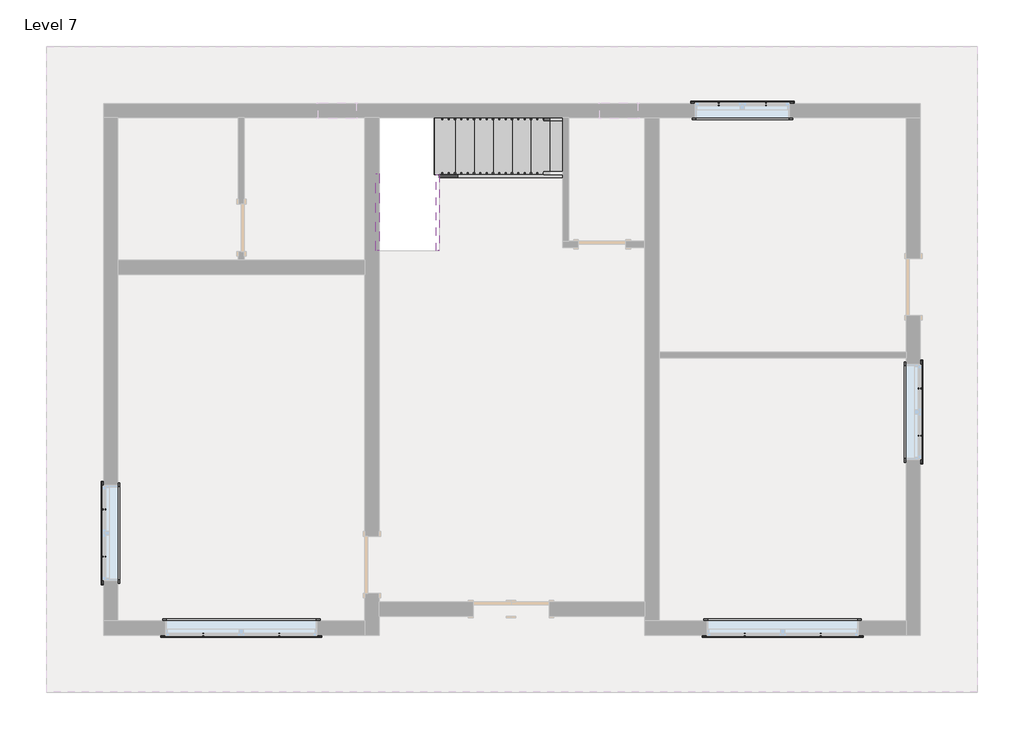
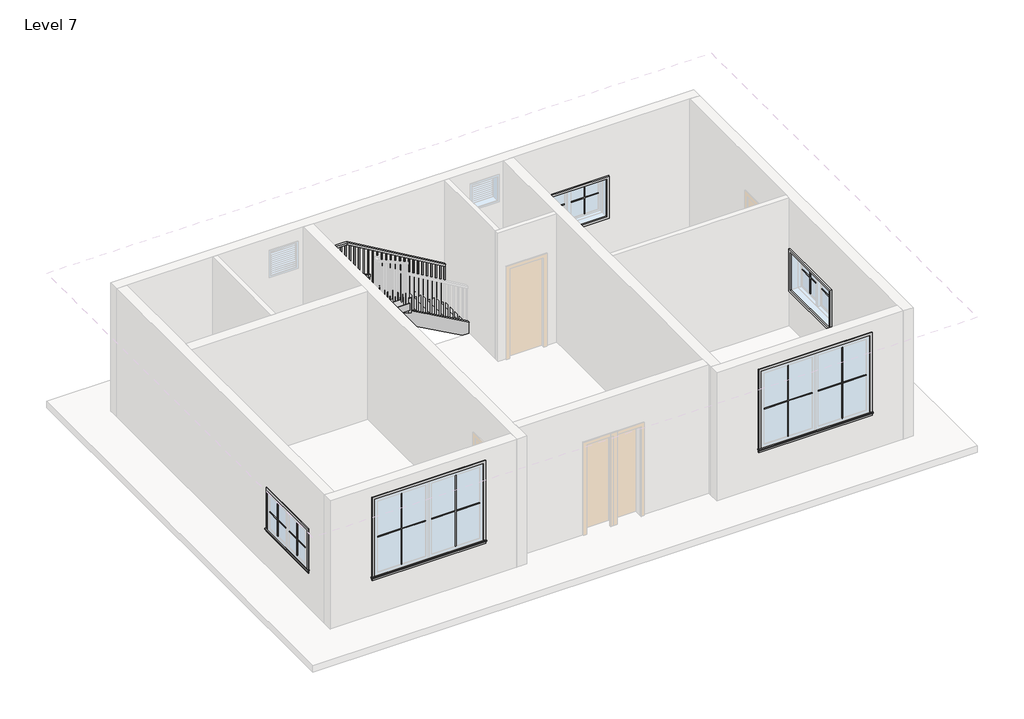
# One storey, part 2 of 2: 20 proxies, 4 members, 1 railing, 1 stair flight.
"""IFC4 building model written with IfcOpenShell, lengths in millimetres."""

from ifc_helpers import new_model, si_unit, frame, origin, place, context, project, spatial, polyline, outline, extrude, faceted_brep, transform, mapped, element, save
from components import muntin_pattern_2x2_muntin_pattern_2x2_9352d081, muntin_pattern_2x2_muntin_pattern_2x2_5c2cbe28, muntin_pattern_2x2_muntin_pattern_2x2_bb8d4d84, muntin_pattern_2x2_muntin_pattern_2x2_d03a1f3c, trim_window_exterior_flat_with_sill_979bde60, trim_window_exterior_flat_with_sill_359ed2ce, trim_window_interior_flat_picture_frame_7883d11b, trim_window_interior_flat_picture_frame_939a8053, stair_flight_890a58f3

model = new_model("IFC4")

# Units and contexts
model_context = context("Model", 3, world=origin())
ifc_project = project(units=[si_unit("LENGTHUNIT", "METRE", prefix="MILLI")], contexts=[model_context])

# Site, building, storey
site = spatial("IfcSite", under=ifc_project)
building = spatial("IfcBuilding", under=site)
storey = spatial("IfcBuildingStorey", under=building, Name="Level 7", Elevation=19050.0)

# Proxies
placement = place(None, origin())
muntin_pattern_2x2_muntin_pattern_2x2_shape = muntin_pattern_2x2_muntin_pattern_2x2_9352d081(model_context)
element("IfcBuildingElementProxy", 1, Name="Muntin Pattern_2x2 : Muntin Pattern_2x2", ObjectType="Muntin Pattern_2x2 : Muntin Pattern_2x2", at=placement, inside=storey, context=model_context, shape_type="MappedRepresentation", body=[
    mapped(muntin_pattern_2x2_muntin_pattern_2x2_shape, transform((-7798.9165084, -1764.5743005, 20034.25), x_axis=(0.0, 1.0, 0.0), y_axis=(-1.0, 0.0, 0.0), z_axis=(0.0, 0.0, 1.0))),
])
element("IfcBuildingElementProxy", 2, Name="Muntin Pattern_2x2 : Muntin Pattern_2x2", ObjectType="Muntin Pattern_2x2 : Muntin Pattern_2x2", at=placement, inside=storey, context=model_context, shape_type="MappedRepresentation", body=[
    mapped(muntin_pattern_2x2_muntin_pattern_2x2_shape, transform((5288.4334916, 937.3506995, 20034.25), x_axis=(0.0, -1.0, 0.0), y_axis=(1.0, 0.0, 0.0), z_axis=(0.0, 0.0, 1.0))),
])
element("IfcBuildingElementProxy", 3, Name="Muntin Pattern_2x2 : Muntin Pattern_2x2", ObjectType="Muntin Pattern_2x2 : Muntin Pattern_2x2", at=placement, inside=storey, context=model_context, shape_type="MappedRepresentation", body=[
    mapped(muntin_pattern_2x2_muntin_pattern_2x2_shape, transform((2061.0459916, 5501.4131995, 20034.25), x_axis=(1.0, 0.0, 0.0), y_axis=(0.0, 1.0, 0.0), z_axis=(0.0, 0.0, 1.0))),
])
muntin_pattern_2x2_muntin_pattern_2x2_2_shape = muntin_pattern_2x2_muntin_pattern_2x2_5c2cbe28(model_context)
element("IfcBuildingElementProxy", 4, Name="Muntin Pattern_2x2 : Muntin Pattern_2x2", ObjectType="Muntin Pattern_2x2 : Muntin Pattern_2x2", at=placement, inside=storey, context=model_context, shape_type="MappedRepresentation", body=[
    mapped(muntin_pattern_2x2_muntin_pattern_2x2_2_shape, transform((-7798.9165084, -1005.7493005, 20034.25), x_axis=(0.0, -1.0, 0.0), y_axis=(1.0, 0.0, 0.0), z_axis=(0.0, 0.0, 1.0))),
])
element("IfcBuildingElementProxy", 5, Name="Muntin Pattern_2x2 : Muntin Pattern_2x2", ObjectType="Muntin Pattern_2x2 : Muntin Pattern_2x2", at=placement, inside=storey, context=model_context, shape_type="MappedRepresentation", body=[
    mapped(muntin_pattern_2x2_muntin_pattern_2x2_2_shape, transform((5288.4334916, 178.5256995, 20034.25), x_axis=(0.0, 1.0, 0.0), y_axis=(-1.0, 0.0, 0.0), z_axis=(0.0, 0.0, 1.0))),
])
element("IfcBuildingElementProxy", 6, Name="Muntin Pattern_2x2 : Muntin Pattern_2x2", ObjectType="Muntin Pattern_2x2 : Muntin Pattern_2x2", at=placement, inside=storey, context=model_context, shape_type="MappedRepresentation", body=[
    mapped(muntin_pattern_2x2_muntin_pattern_2x2_2_shape, transform((2819.8709916, 5501.4131995, 20034.25), x_axis=(-1.0, 0.0, 0.0), y_axis=(0.0, -1.0, 0.0), z_axis=(0.0, 0.0, 1.0))),
])
muntin_pattern_2x2_muntin_pattern_2x2_3_shape = muntin_pattern_2x2_muntin_pattern_2x2_bb8d4d84(model_context)
element("IfcBuildingElementProxy", 7, Name="Muntin Pattern_2x2 : Muntin Pattern_2x2", ObjectType="Muntin Pattern_2x2 : Muntin Pattern_2x2", at=placement, inside=storey, context=model_context, shape_type="MappedRepresentation", body=[
    mapped(muntin_pattern_2x2_muntin_pattern_2x2_3_shape, transform((-4990.6290084, -3013.9368005, 20034.25), x_axis=(-1.0, 0.0, 0.0), y_axis=(0.0, -1.0, 0.0), z_axis=(0.0, 0.0, 1.0))),
])
element("IfcBuildingElementProxy", 8, Name="Muntin Pattern_2x2 : Muntin Pattern_2x2", ObjectType="Muntin Pattern_2x2 : Muntin Pattern_2x2", at=placement, inside=storey, context=model_context, shape_type="MappedRepresentation", body=[
    mapped(muntin_pattern_2x2_muntin_pattern_2x2_3_shape, transform((3696.1709916, -3013.9368005, 20034.25), x_axis=(-1.0, 0.0, 0.0), y_axis=(0.0, -1.0, 0.0), z_axis=(0.0, 0.0, 1.0))),
])
muntin_pattern_2x2_muntin_pattern_2x2_4_shape = muntin_pattern_2x2_muntin_pattern_2x2_d03a1f3c(model_context)
element("IfcBuildingElementProxy", 9, Name="Muntin Pattern_2x2 : Muntin Pattern_2x2", ObjectType="Muntin Pattern_2x2 : Muntin Pattern_2x2", at=placement, inside=storey, context=model_context, shape_type="MappedRepresentation", body=[
    mapped(muntin_pattern_2x2_muntin_pattern_2x2_4_shape, transform((-6206.6540084, -3013.9368005, 20034.25), x_axis=(1.0, 0.0, 0.0), y_axis=(0.0, 1.0, 0.0), z_axis=(0.0, 0.0, 1.0))),
])
element("IfcBuildingElementProxy", 10, Name="Muntin Pattern_2x2 : Muntin Pattern_2x2", ObjectType="Muntin Pattern_2x2 : Muntin Pattern_2x2", at=placement, inside=storey, context=model_context, shape_type="MappedRepresentation", body=[
    mapped(muntin_pattern_2x2_muntin_pattern_2x2_4_shape, transform((2480.1459916, -3013.9368005, 20034.25), x_axis=(1.0, 0.0, 0.0), y_axis=(0.0, 1.0, 0.0), z_axis=(0.0, 0.0, 1.0))),
])
trim_window_exterior_flat_with_sill_shape = trim_window_exterior_flat_with_sill_979bde60(model_context)
element("IfcBuildingElementProxy", 11, Name="Trim-Window-Exterior-Flat : with Sill", ObjectType="Trim-Window-Exterior-Flat : with Sill", at=placement, inside=storey, context=model_context, shape_type="MappedRepresentation", body=[
    mapped(trim_window_exterior_flat_with_sill_shape, transform((-7808.4415084, -1385.1618005, 20878.8), x_axis=(0.0, -1.0, 0.0), y_axis=(0.0, 0.0, 1.0), z_axis=(-1.0, 0.0, 0.0))),
])
element("IfcBuildingElementProxy", 12, Name="Trim-Window-Exterior-Flat : with Sill", ObjectType="Trim-Window-Exterior-Flat : with Sill", at=placement, inside=storey, context=model_context, shape_type="MappedRepresentation", body=[
    mapped(trim_window_exterior_flat_with_sill_shape, transform((5297.9584916, 557.9381995, 20878.8), x_axis=(0.0, 1.0, 0.0), y_axis=(0.0, 0.0, 1.0), z_axis=(1.0, 0.0, 0.0))),
])
element("IfcBuildingElementProxy", 13, Name="Trim-Window-Exterior-Flat : with Sill", ObjectType="Trim-Window-Exterior-Flat : with Sill", at=placement, inside=storey, context=model_context, shape_type="MappedRepresentation", body=[
    mapped(trim_window_exterior_flat_with_sill_shape, transform((2440.4584916, 5510.9381995, 20878.8), x_axis=(-1.0, 0.0, 0.0), y_axis=(0.0, 0.0, 1.0), z_axis=(0.0, 1.0, 0.0))),
])
trim_window_exterior_flat_with_sill_2_shape = trim_window_exterior_flat_with_sill_359ed2ce(model_context)
element("IfcBuildingElementProxy", 14, Name="Trim-Window-Exterior-Flat : with Sill", ObjectType="Trim-Window-Exterior-Flat : with Sill", at=placement, inside=storey, context=model_context, shape_type="MappedRepresentation", body=[
    mapped(trim_window_exterior_flat_with_sill_2_shape, transform((-5598.6415084, -3023.4618005, 21793.2), x_axis=(1.0, 0.0, 0.0), y_axis=(0.0, 0.0, 1.0), z_axis=(0.0, -1.0, 0.0))),
])
element("IfcBuildingElementProxy", 15, Name="Trim-Window-Exterior-Flat : with Sill", ObjectType="Trim-Window-Exterior-Flat : with Sill", at=placement, inside=storey, context=model_context, shape_type="MappedRepresentation", body=[
    mapped(trim_window_exterior_flat_with_sill_2_shape, transform((3088.1584916, -3023.4618005, 21793.2), x_axis=(1.0, 0.0, 0.0), y_axis=(0.0, 0.0, 1.0), z_axis=(0.0, -1.0, 0.0))),
])
trim_window_interior_flat_picture_frame_shape = trim_window_interior_flat_picture_frame_7883d11b(model_context)
element("IfcBuildingElementProxy", 16, Name="Trim-Window-Interior-Flat : Picture Frame", ObjectType="Trim-Window-Interior-Flat : Picture Frame", at=placement, inside=storey, context=model_context, shape_type="MappedRepresentation", body=[
    mapped(trim_window_interior_flat_picture_frame_shape, transform((-7579.8415084, -1385.1618005, 20878.8), x_axis=(0.0, 1.0, 0.0), y_axis=(0.0, 0.0, 1.0), z_axis=(1.0, 0.0, 0.0))),
])
element("IfcBuildingElementProxy", 17, Name="Trim-Window-Interior-Flat : Picture Frame", ObjectType="Trim-Window-Interior-Flat : Picture Frame", at=placement, inside=storey, context=model_context, shape_type="MappedRepresentation", body=[
    mapped(trim_window_interior_flat_picture_frame_shape, transform((5069.3584916, 557.9381995, 20878.8), x_axis=(0.0, -1.0, 0.0), y_axis=(0.0, 0.0, 1.0), z_axis=(-1.0, 0.0, 0.0))),
])
element("IfcBuildingElementProxy", 18, Name="Trim-Window-Interior-Flat : Picture Frame", ObjectType="Trim-Window-Interior-Flat : Picture Frame", at=placement, inside=storey, context=model_context, shape_type="MappedRepresentation", body=[
    mapped(trim_window_interior_flat_picture_frame_shape, transform((2440.4584916, 5282.3381995, 20878.8), x_axis=(1.0, 0.0, 0.0), y_axis=(0.0, 0.0, 1.0), z_axis=(0.0, -1.0, 0.0))),
])
trim_window_interior_flat_picture_frame_2_shape = trim_window_interior_flat_picture_frame_939a8053(model_context)
element("IfcBuildingElementProxy", 19, Name="Trim-Window-Interior-Flat : Picture Frame", ObjectType="Trim-Window-Interior-Flat : Picture Frame", at=placement, inside=storey, context=model_context, shape_type="MappedRepresentation", body=[
    mapped(trim_window_interior_flat_picture_frame_2_shape, transform((-5598.6415084, -2794.8618005, 21793.2), x_axis=(-1.0, 0.0, 0.0), y_axis=(0.0, 0.0, 1.0), z_axis=(0.0, 1.0, 0.0))),
])
element("IfcBuildingElementProxy", 20, Name="Trim-Window-Interior-Flat : Picture Frame", ObjectType="Trim-Window-Interior-Flat : Picture Frame", at=placement, inside=storey, context=model_context, shape_type="MappedRepresentation", body=[
    mapped(trim_window_interior_flat_picture_frame_2_shape, transform((3088.1584916, -2794.8618005, 21793.2), x_axis=(-1.0, 0.0, 0.0), y_axis=(0.0, 0.0, 1.0), z_axis=(0.0, 1.0, 0.0))),
])

# Members
element("IfcMember", 21, ObjectType="Stringer - 2\" Width", at=placement, inside=storey, context=model_context, shape_type="SweptSolid", body=[
    extrude(outline(polyline([(19050.0, -442.4415084), (19314.0428392, -442.4415084), (20414.7095059, -2423.6415084), (20066.0308318, -2423.6415084), (19050.0, -594.7860112), (19050.0, -442.4415084)])), frame((0.0, 4317.5146777, 0.0), z_axis=(0.0, 1.0, 0.0), x_axis=(0.0, 0.0, 1.0)), (0.0, 0.0, 1.0), 50.8),
])
element("IfcMember", 22, ObjectType="Stringer - 2\" Width", at=placement, inside=storey, context=model_context, shape_type="SweptSolid", body=[
    extrude(outline(polyline([(4368.3146777, 20612.245537), (4368.3146777, 20263.6006925), (3148.7383287, 20940.8643411), (3148.7383287, 21289.5091856), (4368.3146777, 20612.245537)])), frame((-2474.4415084, 0.0, 0.0), z_axis=(1.0, 0.0, 0.0), x_axis=(0.0, 1.0, 0.0)), (0.0, 0.0, 1.0), 50.8),
])
element("IfcMember", 23, ObjectType="Stringer - 2\" Width", at=placement, inside=storey, context=model_context, shape_type="SweptSolid", body=[
    extrude(outline(polyline([(19050.0, -442.4415084), (19314.0428392, -442.4415084), (20104.6636166, -1865.5589077), (20104.6636166, -2493.1805211), (19050.0, -594.7860112), (19050.0, -442.4415084)])), frame((0.0, 5282.3381995, 0.0), z_axis=(0.0, 1.0, 0.0), x_axis=(0.0, 0.0, 1.0)), (0.0, 0.0, 1.0), 50.8),
])
element("IfcMember", 24, ObjectType="Stringer - 2\" Width", at=placement, inside=storey, context=model_context, shape_type="SweptSolid", body=[
    extrude(outline(polyline([(3758.489521, 20602.253054), (3148.7383287, 20940.8643411), (3148.7383287, 21289.5091856), (4386.3085505, 20602.253054), (3758.489521, 20602.253054)])), frame((-3439.6415084, 0.0, 0.0), z_axis=(1.0, 0.0, 0.0), x_axis=(0.0, 1.0, 0.0)), (0.0, 0.0, 1.0), 50.8),
])

# Railing
element("IfcRailing", 25, ObjectType="Handrail - Rectangular", at=placement, inside=storey, context=model_context, shape_type="SolidModel", body=[
    faceted_brep([(-442.4415084, 5231.5381995, 20133.7333333), (-442.4415084, 5231.5381995, 20074.9219871), (-442.4415084, 5282.3381995, 20074.9219871), (-442.4415084, 5282.3381995, 20133.7333333), (-2641.0608886, 5231.5381995, 21416.2613051), (-2654.794625, 5231.5381995, 21365.4613051), (-2654.794625, 5282.3381995, 21365.4613051), (-2641.0608886, 5282.3381995, 21416.2613051), (-3338.0415084, 5231.5381995, 21416.2613051), (-3338.0415084, 5231.5381995, 21365.4613051), (-3388.8415084, 5282.3381995, 21365.4613051), (-3388.8415084, 5282.3381995, 21416.2613051), (-3338.0415084, 4498.2044111, 21416.2613051), (-3338.0415084, 4485.04436, 21365.4613051), (-3388.8415084, 4485.04436, 21365.4613051), (-3388.8415084, 4498.2044111, 21416.2613051), (-3338.0415084, 3148.7383287, 22165.7333333), (-3388.8415084, 3148.7383287, 22165.7333333), (-3388.8415084, 3148.7383287, 22107.62445), (-3338.0415084, 3148.7383287, 22107.62445)], [[[0, 1, 2, 3]], [[1, 0, 4, 5]], [[2, 1, 5, 6]], [[3, 2, 6, 7]], [[0, 3, 7, 4]], [[5, 4, 8, 9]], [[6, 5, 9, 10]], [[7, 6, 10, 11]], [[4, 7, 11, 8]], [[9, 8, 12, 13]], [[10, 9, 13, 14]], [[11, 10, 14, 15]], [[8, 11, 15, 12]], [[16, 17, 18, 19]], [[13, 12, 16, 19]], [[14, 13, 19, 18]], [[15, 14, 18, 17]], [[12, 15, 17, 16]]]),
    extrude(outline(polyline([(3215.4131995, 22070.5942858), (3234.4631995, 22060.0142183), (3234.4631995, 21082.0), (3215.4131995, 21082.0), (3215.4131995, 22070.5942858)])), frame((-3372.9665084, 0.0, 0.0), z_axis=(1.0, 0.0, 0.0), x_axis=(0.0, 1.0, 0.0)), (0.0, 0.0, 1.0), 19.05),
    extrude(outline(polyline([(3317.0131995, 22014.3240232), (3336.0631995, 22003.7439558), (3336.0631995, 21082.0), (3317.0131995, 21082.0), (3317.0131995, 22014.3240232)])), frame((-3372.9665084, 0.0, 0.0), z_axis=(1.0, 0.0, 0.0), x_axis=(0.0, 1.0, 0.0)), (0.0, 0.0, 1.0), 19.05),
    extrude(outline(polyline([(3418.6131995, 21957.8969969), (3437.6631995, 21947.3169295), (3437.6631995, 21082.0), (3418.6131995, 21082.0), (3418.6131995, 21957.8969969)])), frame((-3372.9665084, 0.0, 0.0), z_axis=(1.0, 0.0, 0.0), x_axis=(0.0, 1.0, 0.0)), (0.0, 0.0, 1.0), 19.05),
    extrude(outline(polyline([(3520.2131995, 21901.4699707), (3539.2631995, 21890.8899033), (3539.2631995, 20912.6666667), (3520.2131995, 20912.6666667), (3520.2131995, 21901.4699707)])), frame((-3372.9665084, 0.0, 0.0), z_axis=(1.0, 0.0, 0.0), x_axis=(0.0, 1.0, 0.0)), (0.0, 0.0, 1.0), 19.05),
    extrude(outline(polyline([(3621.8131995, 21844.9906899), (3640.8631995, 21834.4106224), (3640.8631995, 20912.6666667), (3621.8131995, 20912.6666667), (3621.8131995, 21844.9906899)])), frame((-3372.9665084, 0.0, 0.0), z_axis=(1.0, 0.0, 0.0), x_axis=(0.0, 1.0, 0.0)), (0.0, 0.0, 1.0), 19.05),
    extrude(outline(polyline([(3723.4131995, 21788.5636636), (3742.4631995, 21777.9835962), (3742.4631995, 20912.6666667), (3723.4131995, 20912.6666667), (3723.4131995, 21788.5636636)])), frame((-3372.9665084, 0.0, 0.0), z_axis=(1.0, 0.0, 0.0), x_axis=(0.0, 1.0, 0.0)), (0.0, 0.0, 1.0), 19.05),
    extrude(outline(polyline([(3825.0131995, 21732.1366374), (3844.0631995, 21721.5565699), (3844.0631995, 20743.3333333), (3825.0131995, 20743.3333333), (3825.0131995, 21732.1366374)])), frame((-3372.9665084, 0.0, 0.0), z_axis=(1.0, 0.0, 0.0), x_axis=(0.0, 1.0, 0.0)), (0.0, 0.0, 1.0), 19.05),
    extrude(outline(polyline([(3926.6131995, 21675.6573565), (3945.6631995, 21665.0772891), (3945.6631995, 20743.3333333), (3926.6131995, 20743.3333333), (3926.6131995, 21675.6573565)])), frame((-3372.9665084, 0.0, 0.0), z_axis=(1.0, 0.0, 0.0), x_axis=(0.0, 1.0, 0.0)), (0.0, 0.0, 1.0), 19.05),
    extrude(outline(polyline([(4028.2131995, 21619.2303303), (4047.2631995, 21608.6502629), (4047.2631995, 20743.3333333), (4028.2131995, 20743.3333333), (4028.2131995, 21619.2303303)])), frame((-3372.9665084, 0.0, 0.0), z_axis=(1.0, 0.0, 0.0), x_axis=(0.0, 1.0, 0.0)), (0.0, 0.0, 1.0), 19.05),
    extrude(outline(polyline([(4129.8131995, 21562.803304), (4148.8631995, 21552.2232366), (4148.8631995, 20574.0), (4129.8131995, 20574.0), (4129.8131995, 21562.803304)])), frame((-3372.9665084, 0.0, 0.0), z_axis=(1.0, 0.0, 0.0), x_axis=(0.0, 1.0, 0.0)), (0.0, 0.0, 1.0), 19.05),
    extrude(outline(polyline([(4231.4131995, 21506.3240232), (4250.4631995, 21495.7439558), (4250.4631995, 20574.0), (4231.4131995, 20574.0), (4231.4131995, 21506.3240232)])), frame((-3372.9665084, 0.0, 0.0), z_axis=(1.0, 0.0, 0.0), x_axis=(0.0, 1.0, 0.0)), (0.0, 0.0, 1.0), 19.05),
    extrude(outline(polyline([(4333.0131995, 21449.8969969), (4352.0631995, 21439.3169295), (4352.0631995, 20574.0), (4333.0131995, 20574.0), (4333.0131995, 21449.8969969)])), frame((-3372.9665084, 0.0, 0.0), z_axis=(1.0, 0.0, 0.0), x_axis=(0.0, 1.0, 0.0)), (0.0, 0.0, 1.0), 19.05),
    extrude(outline(polyline([(4434.6131995, 21393.4699707), (4453.6631995, 21382.8899033), (4453.6631995, 20404.6666667), (4434.6131995, 20404.6666667), (4434.6131995, 21393.4699707)])), frame((-3372.9665084, 0.0, 0.0), z_axis=(1.0, 0.0, 0.0), x_axis=(0.0, 1.0, 0.0)), (0.0, 0.0, 1.0), 19.05),
    extrude(outline(polyline([(-3372.9665084, 4555.2631995), (-3353.9165084, 4555.2631995), (-3353.9165084, 4536.2131995), (-3372.9665084, 4536.2131995), (-3372.9665084, 4555.2631995)])), frame((0.0, 0.0, 20404.6666667), z_axis=(0.0, 0.0, 1.0), x_axis=(1.0, 0.0, 0.0)), (0.0, 0.0, 1.0), 960.7946385),
    extrude(outline(polyline([(-3372.9665084, 4656.8631995), (-3353.9165084, 4656.8631995), (-3353.9165084, 4637.8131995), (-3372.9665084, 4637.8131995), (-3372.9665084, 4656.8631995)])), frame((0.0, 0.0, 20404.6666667), z_axis=(0.0, 0.0, 1.0), x_axis=(1.0, 0.0, 0.0)), (0.0, 0.0, 1.0), 960.7946385),
    extrude(outline(polyline([(-3372.9665084, 4758.4631995), (-3353.9165084, 4758.4631995), (-3353.9165084, 4739.4131995), (-3372.9665084, 4739.4131995), (-3372.9665084, 4758.4631995)])), frame((0.0, 0.0, 20404.6666667), z_axis=(0.0, 0.0, 1.0), x_axis=(1.0, 0.0, 0.0)), (0.0, 0.0, 1.0), 960.7946385),
    extrude(outline(polyline([(-3372.9665084, 4860.0631995), (-3353.9165084, 4860.0631995), (-3353.9165084, 4841.0131995), (-3372.9665084, 4841.0131995), (-3372.9665084, 4860.0631995)])), frame((0.0, 0.0, 20404.6666667), z_axis=(0.0, 0.0, 1.0), x_axis=(1.0, 0.0, 0.0)), (0.0, 0.0, 1.0), 960.7946385),
    extrude(outline(polyline([(-3372.9665084, 4961.6631995), (-3353.9165084, 4961.6631995), (-3353.9165084, 4942.6131995), (-3372.9665084, 4942.6131995), (-3372.9665084, 4961.6631995)])), frame((0.0, 0.0, 20404.6666667), z_axis=(0.0, 0.0, 1.0), x_axis=(1.0, 0.0, 0.0)), (0.0, 0.0, 1.0), 960.7946385),
    extrude(outline(polyline([(-3372.9665084, 5063.2631995), (-3353.9165084, 5063.2631995), (-3353.9165084, 5044.2131995), (-3372.9665084, 5044.2131995), (-3372.9665084, 5063.2631995)])), frame((0.0, 0.0, 20404.6666667), z_axis=(0.0, 0.0, 1.0), x_axis=(1.0, 0.0, 0.0)), (0.0, 0.0, 1.0), 960.7946385),
    extrude(outline(polyline([(-3372.9665084, 5164.8631995), (-3353.9165084, 5164.8631995), (-3353.9165084, 5145.8131995), (-3372.9665084, 5145.8131995), (-3372.9665084, 5164.8631995)])), frame((0.0, 0.0, 20404.6666667), z_axis=(0.0, 0.0, 1.0), x_axis=(1.0, 0.0, 0.0)), (0.0, 0.0, 1.0), 960.7946385),
    extrude(outline(polyline([(-3277.7165084, 5266.4631995), (-3277.7165084, 5247.4131995), (-3296.7665084, 5247.4131995), (-3296.7665084, 5266.4631995), (-3277.7165084, 5266.4631995)])), frame((0.0, 0.0, 20404.6666667), z_axis=(0.0, 0.0, 1.0), x_axis=(1.0, 0.0, 0.0)), (0.0, 0.0, 1.0), 960.7946385),
    extrude(outline(polyline([(-3176.1165084, 5266.4631995), (-3176.1165084, 5247.4131995), (-3195.1665084, 5247.4131995), (-3195.1665084, 5266.4631995), (-3176.1165084, 5266.4631995)])), frame((0.0, 0.0, 20404.6666667), z_axis=(0.0, 0.0, 1.0), x_axis=(1.0, 0.0, 0.0)), (0.0, 0.0, 1.0), 960.7946385),
    extrude(outline(polyline([(-3074.5165084, 5266.4631995), (-3074.5165084, 5247.4131995), (-3093.5665084, 5247.4131995), (-3093.5665084, 5266.4631995), (-3074.5165084, 5266.4631995)])), frame((0.0, 0.0, 20404.6666667), z_axis=(0.0, 0.0, 1.0), x_axis=(1.0, 0.0, 0.0)), (0.0, 0.0, 1.0), 960.7946385),
    extrude(outline(polyline([(-2972.9165084, 5266.4631995), (-2972.9165084, 5247.4131995), (-2991.9665084, 5247.4131995), (-2991.9665084, 5266.4631995), (-2972.9165084, 5266.4631995)])), frame((0.0, 0.0, 20404.6666667), z_axis=(0.0, 0.0, 1.0), x_axis=(1.0, 0.0, 0.0)), (0.0, 0.0, 1.0), 960.7946385),
    extrude(outline(polyline([(-2871.3165084, 5266.4631995), (-2871.3165084, 5247.4131995), (-2890.3665084, 5247.4131995), (-2890.3665084, 5266.4631995), (-2871.3165084, 5266.4631995)])), frame((0.0, 0.0, 20404.6666667), z_axis=(0.0, 0.0, 1.0), x_axis=(1.0, 0.0, 0.0)), (0.0, 0.0, 1.0), 960.7946385),
    extrude(outline(polyline([(-2769.7165084, 5266.4631995), (-2769.7165084, 5247.4131995), (-2788.7665084, 5247.4131995), (-2788.7665084, 5266.4631995), (-2769.7165084, 5266.4631995)])), frame((0.0, 0.0, 20404.6666667), z_axis=(0.0, 0.0, 1.0), x_axis=(1.0, 0.0, 0.0)), (0.0, 0.0, 1.0), 960.7946385),
    extrude(outline(polyline([(-2668.1165084, 5266.4631995), (-2668.1165084, 5247.4131995), (-2687.1665084, 5247.4131995), (-2687.1665084, 5266.4631995), (-2668.1165084, 5266.4631995)])), frame((0.0, 0.0, 20404.6666667), z_axis=(0.0, 0.0, 1.0), x_axis=(1.0, 0.0, 0.0)), (0.0, 0.0, 1.0), 960.7946385),
    extrude(outline(polyline([(21313.9657371, -2566.5165084), (21325.0782371, -2585.5665084), (20404.6666667, -2585.5665084), (20404.6666667, -2566.5165084), (21313.9657371, -2566.5165084)])), frame((0.0, 5247.4131995, 0.0), z_axis=(0.0, 1.0, 0.0), x_axis=(0.0, 0.0, 1.0)), (0.0, 0.0, 1.0), 19.05),
    extrude(outline(polyline([(21254.6990704, -2464.9165084), (21265.8115704, -2483.9665084), (20404.6666667, -2483.9665084), (20404.6666667, -2464.9165084), (21254.6990704, -2464.9165084)])), frame((0.0, 5247.4131995, 0.0), z_axis=(0.0, 1.0, 0.0), x_axis=(0.0, 0.0, 1.0)), (0.0, 0.0, 1.0), 19.05),
    extrude(outline(polyline([(21195.4324038, -2363.3165084), (21206.5449038, -2382.3665084), (20235.3333333, -2382.3665084), (20235.3333333, -2363.3165084), (21195.4324038, -2363.3165084)])), frame((0.0, 5247.4131995, 0.0), z_axis=(0.0, 1.0, 0.0), x_axis=(0.0, 0.0, 1.0)), (0.0, 0.0, 1.0), 19.05),
    extrude(outline(polyline([(21136.1657371, -2261.7165084), (21147.2782371, -2280.7665084), (20235.3333333, -2280.7665084), (20235.3333333, -2261.7165084), (21136.1657371, -2261.7165084)])), frame((0.0, 5247.4131995, 0.0), z_axis=(0.0, 1.0, 0.0), x_axis=(0.0, 0.0, 1.0)), (0.0, 0.0, 1.0), 19.05),
    extrude(outline(polyline([(21076.8990704, -2160.1165084), (21088.0115704, -2179.1665084), (20235.3333333, -2179.1665084), (20235.3333333, -2160.1165084), (21076.8990704, -2160.1165084)])), frame((0.0, 5247.4131995, 0.0), z_axis=(0.0, 1.0, 0.0), x_axis=(0.0, 0.0, 1.0)), (0.0, 0.0, 1.0), 19.05),
    extrude(outline(polyline([(21017.6324038, -2058.5165084), (21028.7449038, -2077.5665084), (20066.0, -2077.5665084), (20066.0, -2058.5165084), (21017.6324038, -2058.5165084)])), frame((0.0, 5247.4131995, 0.0), z_axis=(0.0, 1.0, 0.0), x_axis=(0.0, 0.0, 1.0)), (0.0, 0.0, 1.0), 19.05),
    extrude(outline(polyline([(20958.3657371, -1956.9165084), (20969.4782371, -1975.9665084), (20066.0, -1975.9665084), (20066.0, -1956.9165084), (20958.3657371, -1956.9165084)])), frame((0.0, 5247.4131995, 0.0), z_axis=(0.0, 1.0, 0.0), x_axis=(0.0, 0.0, 1.0)), (0.0, 0.0, 1.0), 19.05),
    extrude(outline(polyline([(20899.0990704, -1855.3165084), (20910.2115704, -1874.3665084), (20066.0, -1874.3665084), (20066.0, -1855.3165084), (20899.0990704, -1855.3165084)])), frame((0.0, 5247.4131995, 0.0), z_axis=(0.0, 1.0, 0.0), x_axis=(0.0, 0.0, 1.0)), (0.0, 0.0, 1.0), 19.05),
    extrude(outline(polyline([(20839.8324038, -1753.7165084), (20850.9449038, -1772.7665084), (19896.6666667, -1772.7665084), (19896.6666667, -1753.7165084), (20839.8324038, -1753.7165084)])), frame((0.0, 5247.4131995, 0.0), z_axis=(0.0, 1.0, 0.0), x_axis=(0.0, 0.0, 1.0)), (0.0, 0.0, 1.0), 19.05),
    extrude(outline(polyline([(20780.5657371, -1652.1165084), (20791.6782371, -1671.1665084), (19896.6666667, -1671.1665084), (19896.6666667, -1652.1165084), (20780.5657371, -1652.1165084)])), frame((0.0, 5247.4131995, 0.0), z_axis=(0.0, 1.0, 0.0), x_axis=(0.0, 0.0, 1.0)), (0.0, 0.0, 1.0), 19.05),
    extrude(outline(polyline([(20721.2990704, -1550.5165084), (20732.4115704, -1569.5665084), (19896.6666667, -1569.5665084), (19896.6666667, -1550.5165084), (20721.2990704, -1550.5165084)])), frame((0.0, 5247.4131995, 0.0), z_axis=(0.0, 1.0, 0.0), x_axis=(0.0, 0.0, 1.0)), (0.0, 0.0, 1.0), 19.05),
    extrude(outline(polyline([(20662.0324038, -1448.9165084), (20673.1449038, -1467.9665084), (19727.3333333, -1467.9665084), (19727.3333333, -1448.9165084), (20662.0324038, -1448.9165084)])), frame((0.0, 5247.4131995, 0.0), z_axis=(0.0, 1.0, 0.0), x_axis=(0.0, 0.0, 1.0)), (0.0, 0.0, 1.0), 19.05),
    extrude(outline(polyline([(20602.7657371, -1347.3165084), (20613.8782371, -1366.3665084), (19727.3333333, -1366.3665084), (19727.3333333, -1347.3165084), (20602.7657371, -1347.3165084)])), frame((0.0, 5247.4131995, 0.0), z_axis=(0.0, 1.0, 0.0), x_axis=(0.0, 0.0, 1.0)), (0.0, 0.0, 1.0), 19.05),
    extrude(outline(polyline([(20543.4990704, -1245.7165084), (20554.6115704, -1264.7665084), (19727.3333333, -1264.7665084), (19727.3333333, -1245.7165084), (20543.4990704, -1245.7165084)])), frame((0.0, 5247.4131995, 0.0), z_axis=(0.0, 1.0, 0.0), x_axis=(0.0, 0.0, 1.0)), (0.0, 0.0, 1.0), 19.05),
    extrude(outline(polyline([(20484.2324038, -1144.1165084), (20495.3449038, -1163.1665084), (19558.0, -1163.1665084), (19558.0, -1144.1165084), (20484.2324038, -1144.1165084)])), frame((0.0, 5247.4131995, 0.0), z_axis=(0.0, 1.0, 0.0), x_axis=(0.0, 0.0, 1.0)), (0.0, 0.0, 1.0), 19.05),
    extrude(outline(polyline([(20424.9657371, -1042.5165084), (20436.0782371, -1061.5665084), (19558.0, -1061.5665084), (19558.0, -1042.5165084), (20424.9657371, -1042.5165084)])), frame((0.0, 5247.4131995, 0.0), z_axis=(0.0, 1.0, 0.0), x_axis=(0.0, 0.0, 1.0)), (0.0, 0.0, 1.0), 19.05),
    extrude(outline(polyline([(20365.6990704, -940.9165084), (20376.8115704, -959.9665084), (19558.0, -959.9665084), (19558.0, -940.9165084), (20365.6990704, -940.9165084)])), frame((0.0, 5247.4131995, 0.0), z_axis=(0.0, 1.0, 0.0), x_axis=(0.0, 0.0, 1.0)), (0.0, 0.0, 1.0), 19.05),
    extrude(outline(polyline([(20306.4324038, -839.3165084), (20317.5449038, -858.3665084), (19388.6666667, -858.3665084), (19388.6666667, -839.3165084), (20306.4324038, -839.3165084)])), frame((0.0, 5247.4131995, 0.0), z_axis=(0.0, 1.0, 0.0), x_axis=(0.0, 0.0, 1.0)), (0.0, 0.0, 1.0), 19.05),
    extrude(outline(polyline([(20247.1657371, -737.7165084), (20258.2782371, -756.7665084), (19388.6666667, -756.7665084), (19388.6666667, -737.7165084), (20247.1657371, -737.7165084)])), frame((0.0, 5247.4131995, 0.0), z_axis=(0.0, 1.0, 0.0), x_axis=(0.0, 0.0, 1.0)), (0.0, 0.0, 1.0), 19.05),
    extrude(outline(polyline([(20187.8990704, -636.1165084), (20199.0115704, -655.1665084), (19388.6666667, -655.1665084), (19388.6666667, -636.1165084), (20187.8990704, -636.1165084)])), frame((0.0, 5247.4131995, 0.0), z_axis=(0.0, 1.0, 0.0), x_axis=(0.0, 0.0, 1.0)), (0.0, 0.0, 1.0), 19.05),
    extrude(outline(polyline([(20128.6324038, -534.5165084), (20139.7449038, -553.5665084), (19219.3333333, -553.5665084), (19219.3333333, -534.5165084), (20128.6324038, -534.5165084)])), frame((0.0, 5247.4131995, 0.0), z_axis=(0.0, 1.0, 0.0), x_axis=(0.0, 0.0, 1.0)), (0.0, 0.0, 1.0), 19.05),
    extrude(outline(polyline([(-3353.9165084, 5266.4631995), (-3353.9165084, 5247.4131995), (-3372.9665084, 5247.4131995), (-3372.9665084, 5266.4631995), (-3353.9165084, 5266.4631995)])), frame((0.0, 0.0, 20404.6666667), z_axis=(0.0, 0.0, 1.0), x_axis=(1.0, 0.0, 0.0)), (0.0, 0.0, 1.0), 960.7946385),
    extrude(outline(polyline([(3148.7383287, 22107.62445), (3167.7883287, 22097.0443826), (3167.7883287, 21082.0), (3148.7383287, 21082.0), (3148.7383287, 22107.62445)])), frame((-3372.9665084, 0.0, 0.0), z_axis=(1.0, 0.0, 0.0), x_axis=(0.0, 1.0, 0.0)), (0.0, 0.0, 1.0), 19.05),
    extrude(outline(polyline([(20074.9219871, -442.4415084), (20086.0344871, -461.4915084), (19219.3333333, -461.4915084), (19219.3333333, -442.4415084), (20074.9219871, -442.4415084)])), frame((0.0, 5247.4131995, 0.0), z_axis=(0.0, 1.0, 0.0), x_axis=(0.0, 0.0, 1.0)), (0.0, 0.0, 1.0), 19.05),
])

# Stair flight
stair_flight_shape = stair_flight_890a58f3(model_context)
element("IfcStairFlight", 26, ObjectType="2\" Tread 1\" Nosing 1/4\" Riser", at=placement, inside=storey, context=model_context, shape_type="MappedRepresentation", body=[
    mapped(stair_flight_shape, transform((0.0, 0.0, 0.0), x_axis=(1.0, 0.0, 0.0), y_axis=(0.0, 1.0, 0.0), z_axis=(0.0, 0.0, 1.0))),
])

save(model, "model.ifc")

# Revit data of these elements
# Type "Muntin Pattern_2x2 : Muntin Pattern_2x2"
#   Width [instance default] = 4' - 0"
#   Thickness = 0' - 0 1/2"
#   Height [instance default] = 4' - 0"
#   Distance = 0' - 0 3/4"
#   Interior Material [instance default] = none
#   Exterior Material [instance default] = none
#   Default Elevation = 0
# Type "Trim-Window-Exterior-Flat : with Sill"
#   Trim Width = 0' - 2 1/4"
#   Trim Thickness_Picture Frame = 0' - 1 1/4"
#   Trim Thickness_with Sill = 0' - 0 3/4"
#   Sill Thickness = 0' - 1 1/4"
#   Opening Width [instance default] = 2' - 0"
#   Opening Height [instance default] = 3' - 0"
#   Default Elevation = 4' - 0"
#   Sill = yes
#   Picture Frame = no
#   Trim Material [instance default] = none
# Type "Trim-Window-Interior-Flat : Picture Frame"
#   Trim Thickness_Picture Frame = 0' - 1 1/4"
#   Trim Width = 0' - 2 1/4"
#   Trim Thickness_with Sill = 0' - 0 3/4"
#   Sill Thickness = 0' - 1 1/4"
#   Opening Width [instance default] = 2' - 0"
#   Opening Height [instance default] = 3' - 0"
#   Default Elevation = 4' - 0"
#   Sill = no
#   Picture Frame = yes
#   Trim Material [instance default] = none
# Type "Handrail - Rectangular"
#   Assembly Code = "C2010400"
#   built-in parameter 1008612 = 0.0416667 (stored number, unit not read)
#   built-in parameter 1008611 = 0.0416667 (stored number, unit not read)
#   built-in parameter 1008609 = 0.333333 (stored number, unit not read)
#   built-in parameter 1008604 = 0.166667 (stored number, unit not read)
#   built-in parameter 1008603 = 0.166667 (stored number, unit not read)
#   Railing Height = 3' - 0"
#   built-in parameter 1008630 = 2
#   built-in parameter 1008610 = 2
#   built-in parameter 1008618 = Baluster - Square : 3/4"
# Elements 1, 2, 3, 4, 5, 6 (IfcBuildingElementProxy, "Muntin Pattern_2x2 : Muntin Pattern_2x2")
#   Width = 2' - 0 5/8"
#   Height = 2' - 6 1/2"
#   Interior Material = Wood - Stained
#   Exterior Material = Clad - White
#   Phase Created = New Construction
#   Materials on its faces: "Clad - White", "Wood - Stained"
# Elements 7, 8, 9, 10 (IfcBuildingElementProxy, "Muntin Pattern_2x2 : Muntin Pattern_2x2")
#   Width = 3' - 6 5/8"
#   Height = 5' - 6 1/2"
#   Interior Material = Wood - Stained
#   Exterior Material = Clad - White
#   Phase Created = New Construction
#   Materials on its faces: "Clad - White", "Wood - Stained"
# Elements 11, 12, 13 (IfcBuildingElementProxy, "Trim-Window-Exterior-Flat : with Sill")
#   Opening Width = 5' - 0"
#   Opening Height = 3' - 0"
#   Trim Material = Clad - White
#   Phase Created = New Construction
#   Materials on its faces: "Clad - White"
# Elements 14, 15 (IfcBuildingElementProxy, "Trim-Window-Exterior-Flat : with Sill")
#   Opening Width = 8' - 0"
#   Opening Height = 6' - 0"
#   Trim Material = Clad - White
#   Phase Created = New Construction
#   Materials on its faces: "Clad - White"
# Elements 16, 17, 18 (IfcBuildingElementProxy, "Trim-Window-Interior-Flat : Picture Frame")
#   Opening Width = 5' - 0"
#   Opening Height = 3' - 0"
#   Trim Material = Wood - Stained
#   Phase Created = New Construction
#   Materials on its faces: "Wood - Stained"
# Elements 19, 20 (IfcBuildingElementProxy, "Trim-Window-Interior-Flat : Picture Frame")
#   Opening Width = 8' - 0"
#   Opening Height = 6' - 0"
#   Trim Material = Wood - Stained
#   Phase Created = New Construction
#   Materials on its faces: "Wood - Stained"
# Elements 21, 22, 23, 24 (IfcMember, "Stringer - 2\" Width")
#   Phase Created = New Construction
# Element 25 (IfcRailing, "Handrail - Rectangular")
#   Phase Created = New Construction
# Element 26 (IfcStairFlight, "2\" Tread 1\" Nosing 1/4\" Riser")
#   Phase Created = New Construction
# Materials
#   "Clad - White": class "Wood", colour RGB 242 242 238, transparency 0, Cost = 0
#   "Wood - Stained": class "Wood", colour RGB 224 178 126, transparency 0, Cost = 0
